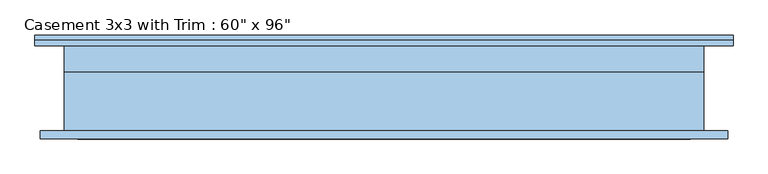
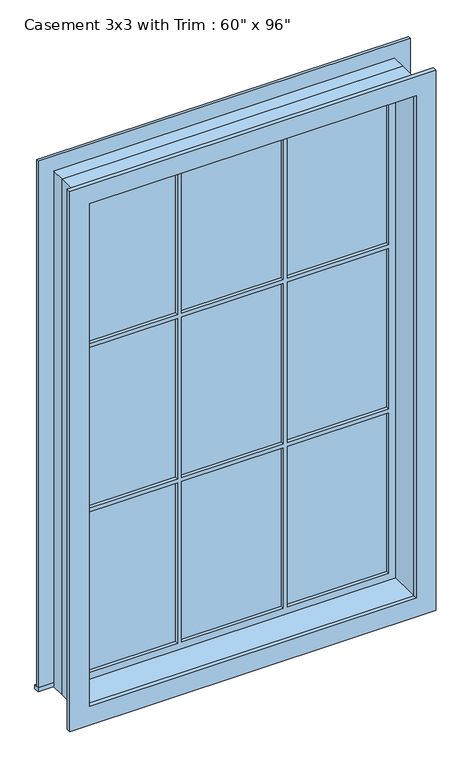
"""IFC4 building model written with IfcOpenShell, lengths in millimetres: window geometry."""

from ifc_helpers import new_model, si_unit, frame, origin, place, context, project, spatial, polyline, outline, extrude, source, transform, mapped, element, save


def window_41dcc157(model_context):
    return source(origin(), model_context, "Body", "SweptSolid", [
        extrude(outline(polyline([(-831.85, 127.0), (831.85, 127.0), (831.85, 101.6), (-831.85, 101.6), (-831.85, 127.0)])), frame((0.0, 0.0, 304.8), z_axis=(0.0, 0.0, 1.0), x_axis=(1.0, 0.0, 0.0)), (0.0, 0.0, 1.0), 19.05),
        extrude(outline(polyline([(2724.15, -742.95), (2724.15, 742.95), (323.85, 742.95), (323.85, 831.85), (2813.05, 831.85), (2813.05, -831.85), (323.85, -831.85), (323.85, -742.95), (2724.15, -742.95)])), frame((0.0, 101.6, 0.0), z_axis=(0.0, 1.0, 0.0), x_axis=(0.0, 0.0, 1.0)), (0.0, 0.0, 1.0), 12.7),
        extrude(outline(polyline([(245.5333333, 66.675), (698.5, 66.675), (698.5, 53.975), (245.5333333, 53.975), (245.5333333, 66.675)])), frame((0.0, 0.0, 1921.9333333), z_axis=(0.0, 0.0, 1.0), x_axis=(1.0, 0.0, 0.0)), (0.0, 0.0, 1.0), 757.7666667),
        extrude(outline(polyline([(-226.4833333, 66.675), (226.4833333, 66.675), (226.4833333, 53.975), (-226.4833333, 53.975), (-226.4833333, 66.675)])), frame((0.0, 0.0, 1921.9333333), z_axis=(0.0, 0.0, 1.0), x_axis=(1.0, 0.0, 0.0)), (0.0, 0.0, 1.0), 757.7666667),
        extrude(outline(polyline([(-698.5, 66.675), (-245.5333333, 66.675), (-245.5333333, 53.975), (-698.5, 53.975), (-698.5, 66.675)])), frame((0.0, 0.0, 1921.9333333), z_axis=(0.0, 0.0, 1.0), x_axis=(1.0, 0.0, 0.0)), (0.0, 0.0, 1.0), 757.7666667),
        extrude(outline(polyline([(-698.5, 66.675), (-245.5333333, 66.675), (-245.5333333, 53.975), (-698.5, 53.975), (-698.5, 66.675)])), frame((0.0, 0.0, 1145.1166667), z_axis=(0.0, 0.0, 1.0), x_axis=(1.0, 0.0, 0.0)), (0.0, 0.0, 1.0), 757.7666667),
        extrude(outline(polyline([(-226.4833333, 66.675), (226.4833333, 66.675), (226.4833333, 53.975), (-226.4833333, 53.975), (-226.4833333, 66.675)])), frame((0.0, 0.0, 1145.1166667), z_axis=(0.0, 0.0, 1.0), x_axis=(1.0, 0.0, 0.0)), (0.0, 0.0, 1.0), 757.7666667),
        extrude(outline(polyline([(245.5333333, 66.675), (698.5, 66.675), (698.5, 53.975), (245.5333333, 53.975), (245.5333333, 66.675)])), frame((0.0, 0.0, 1145.1166667), z_axis=(0.0, 0.0, 1.0), x_axis=(1.0, 0.0, 0.0)), (0.0, 0.0, 1.0), 757.7666667),
        extrude(outline(polyline([(245.5333333, 66.675), (698.5, 66.675), (698.5, 53.975), (245.5333333, 53.975), (245.5333333, 66.675)])), frame((0.0, 0.0, 368.3), z_axis=(0.0, 0.0, 1.0), x_axis=(1.0, 0.0, 0.0)), (0.0, 0.0, 1.0), 757.7666667),
        extrude(outline(polyline([(-226.4833333, 66.675), (226.4833333, 66.675), (226.4833333, 53.975), (-226.4833333, 53.975), (-226.4833333, 66.675)])), frame((0.0, 0.0, 368.3), z_axis=(0.0, 0.0, 1.0), x_axis=(1.0, 0.0, 0.0)), (0.0, 0.0, 1.0), 757.7666667),
        extrude(outline(polyline([(-698.5, 66.675), (-245.5333333, 66.675), (-245.5333333, 53.975), (-698.5, 53.975), (-698.5, 66.675)])), frame((0.0, 0.0, 368.3), z_axis=(0.0, 0.0, 1.0), x_axis=(1.0, 0.0, 0.0)), (0.0, 0.0, 1.0), 757.7666667),
        extrude(outline(polyline([(2800.35, 819.15), (2800.35, -819.15), (247.65, -819.15), (247.65, 819.15), (2800.35, 819.15)]), holes=[polyline([(2711.45, 730.25), (336.55, 730.25), (336.55, -730.25), (2711.45, -730.25), (2711.45, 730.25)])]), frame((0.0, -120.65, 0.0), z_axis=(0.0, 1.0, 0.0), x_axis=(0.0, 0.0, 1.0)), (0.0, 0.0, 1.0), 19.05),
        extrude(outline(polyline([(2724.15, -742.95), (323.85, -742.95), (323.85, 742.95), (2724.15, 742.95), (2724.15, -742.95)]), holes=[polyline([(2679.7, -245.5333333), (1921.9333333, -245.5333333), (1921.9333333, -698.5), (2679.7, -698.5), (2679.7, -245.5333333)]), polyline([(1902.8833333, -245.5333333), (1145.1166667, -245.5333333), (1145.1166667, -698.5), (1902.8833333, -698.5), (1902.8833333, -245.5333333)]), polyline([(1126.0666667, -245.5333333), (368.3, -245.5333333), (368.3, -698.5), (1126.0666667, -698.5), (1126.0666667, -245.5333333)]), polyline([(2679.7, 226.4833333), (1921.9333333, 226.4833333), (1921.9333333, -226.4833333), (2679.7, -226.4833333), (2679.7, 226.4833333)]), polyline([(1902.8833333, 226.4833333), (1145.1166667, 226.4833333), (1145.1166667, -226.4833333), (1902.8833333, -226.4833333), (1902.8833333, 226.4833333)]), polyline([(1126.0666667, 226.4833333), (368.3, 226.4833333), (368.3, -226.4833333), (1126.0666667, -226.4833333), (1126.0666667, 226.4833333)]), polyline([(2679.7, 698.5), (1921.9333333, 698.5), (1921.9333333, 245.5333333), (2679.7, 245.5333333), (2679.7, 698.5)]), polyline([(1902.8833333, 698.5), (1145.1166667, 698.5), (1145.1166667, 245.5333333), (1902.8833333, 245.5333333), (1902.8833333, 698.5)]), polyline([(1126.0666667, 698.5), (368.3, 698.5), (368.3, 245.5333333), (1126.0666667, 245.5333333), (1126.0666667, 698.5)])]), frame((0.0, 38.1, 0.0), z_axis=(0.0, 1.0, 0.0), x_axis=(0.0, 0.0, 1.0)), (0.0, 0.0, 1.0), 44.45),
        extrude(outline(polyline([(2743.2, -762.0), (304.8, -762.0), (304.8, 762.0), (2743.2, 762.0), (2743.2, -762.0)]), holes=[polyline([(2711.45, -730.25), (2711.45, 730.25), (336.55, 730.25), (336.55, -730.25), (2711.45, -730.25)])]), frame((0.0, -101.6, 0.0), z_axis=(0.0, 1.0, 0.0), x_axis=(0.0, 0.0, 1.0)), (0.0, 0.0, 1.0), 139.7),
        extrude(outline(polyline([(2743.2, 762.0), (2743.2, -762.0), (304.8, -762.0), (304.8, 762.0), (2743.2, 762.0)]), holes=[polyline([(2724.15, 742.95), (323.85, 742.95), (323.85, -742.95), (2724.15, -742.95), (2724.15, 742.95)])]), frame((0.0, 38.1, 0.0), z_axis=(0.0, 1.0, 0.0), x_axis=(0.0, 0.0, 1.0)), (0.0, 0.0, 1.0), 63.5),
    ])


if __name__ == "__main__":
    model = new_model("IFC4")
    model_context = context("Model", 3, world=origin())
    ifc_project = project(units=[si_unit("LENGTHUNIT", "METRE", prefix="MILLI")], contexts=[model_context])
    site = spatial("IfcSite", under=ifc_project)
    building = spatial("IfcBuilding", under=site)
    placement = place(None, origin())
    window_shape = window_41dcc157(model_context)
    element("IfcWindow", 1, ObjectType="Casement 3x3 with Trim : 60\" x 96\"", at=placement, inside=building, context=model_context, shape_type="MappedRepresentation", body=[
        mapped(window_shape, transform((0.0, 0.0, 0.0), x_axis=(1.0, 0.0, 0.0), y_axis=(0.0, 1.0, 0.0), z_axis=(0.0, 0.0, 1.0))),
    ])
    save(model, "model.ifc")

# Revit data of these elements
# Type "Casement 3x3 with Trim : 60\" x 96\""
#   Type Mark = "15"
#   Construction Type Id = "GSP4R"
#   Assembly Code = "B2020100"
#   Analytic Construction = "1/8 in Pilkington single glazing"
#   Visual Light Transmittance = 0.9
#   Solar Heat Gain Coefficient = 0.78
#   Heat Transfer Coefficient (U) = 0.6496 BTU/(h·ft²·°F)
#   Height = 8' - 0"
#   Default Sill Height = 1' - 0"
#   Trim Projection - Ext. = 0' - 0 1/2"
#   Trim Projection - Int. = 0' - 0 3/4"
#   Trim Width - Exterior = 0' - 3 1/2"
#   Trim Width - Interior = 0' - 3 1/2"
#   Width = 5' - 0"
#   Window Inset = 0' - 0 3/4"
#   Define Thermal Properties by = 1
#   Glass Pane Material = Glass
#   Sash Material = Sash
#   Trim Exterior Material = Trim
#   Trim Interior Material = Trim
#   Wall Closure = (empty or 0)
# Element 1 (IfcWindow, "Casement 3x3 with Trim : 60\" x 96\"")
#   Materials on its faces: "Sash", "Glass", "Trim"
# Materials
#   "Glass": class "Glass", colour RGB 0 128 192, transparency 0.75, Description = "Soda Lime Glass", Cost = 0
#   "Sash": class "Wood", colour RGB 224 178 126, transparency 0
#   "Trim": class "Wood", colour RGB 224 178 126, transparency 0
